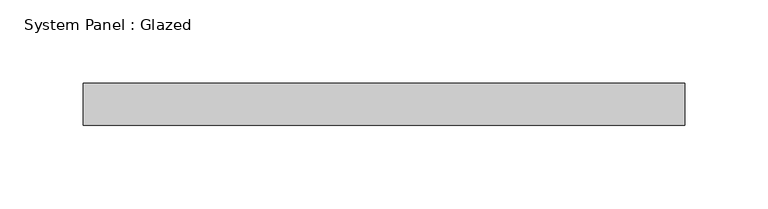
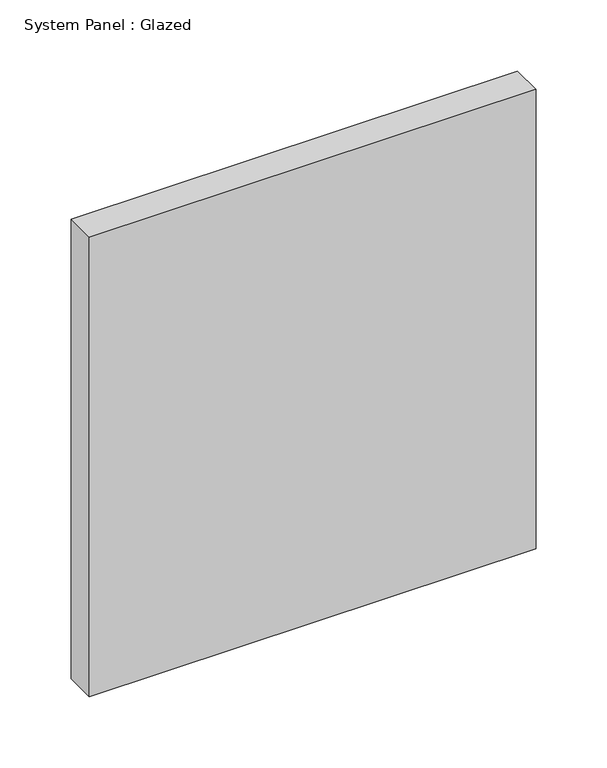
"""IFC4 building model written with IfcOpenShell, lengths in millimetres: plate geometry, System Panel : Glazed."""

from ifc_helpers import new_model, si_unit, origin, origin_with_axes, place, context, project, spatial, polyline, outline, extrude, source, transform, mapped, element, save


def system_panel_glazed_b220ba01(model_context):
    return source(origin(), model_context, "Body", "SweptSolid", [
        extrude(outline(polyline([(180.975, 19.05), (-180.975, 19.05), (-180.975, 44.45), (180.975, 44.45), (180.975, 19.05)])), origin_with_axes(), (0.0, 0.0, 1.0), 393.7),
    ])


if __name__ == "__main__":
    model = new_model("IFC4")
    model_context = context("Model", 3, world=origin())
    ifc_project = project(units=[si_unit("LENGTHUNIT", "METRE", prefix="MILLI")], contexts=[model_context])
    site = spatial("IfcSite", under=ifc_project)
    building = spatial("IfcBuilding", under=site)
    placement = place(None, origin())
    system_panel_glazed_shape = system_panel_glazed_b220ba01(model_context)
    element("IfcPlate", 1, ObjectType="System Panel : Glazed", at=placement, inside=building, context=model_context, shape_type="MappedRepresentation", body=[
        mapped(system_panel_glazed_shape, transform((0.0, 0.0, 0.0), x_axis=(1.0, 0.0, 0.0), y_axis=(0.0, 1.0, 0.0), z_axis=(0.0, 0.0, 1.0))),
    ])
    save(model, "model.ifc")

# Revit data of these elements
# Type "System Panel : Glazed"
#   Construction Type Id = "GSP4R"
#   Analytic Construction = "1/8 in Pilkington single glazing"
#   Visual Light Transmittance = 0.9
#   Solar Heat Gain Coefficient = 0.86
#   Heat Transfer Coefficient (U) = 1.18115 BTU/(h·ft²·°F)
#   Define Thermal Properties by = 1
# Element 1 (IfcPlate, "System Panel : Glazed")
#   Materials on its faces: "Glass"
# Materials
#   "Glass": class "Glass", colour RGB 0 128 192, transparency 0.75, Description = "Soda Lime Glass", Cost = 0
